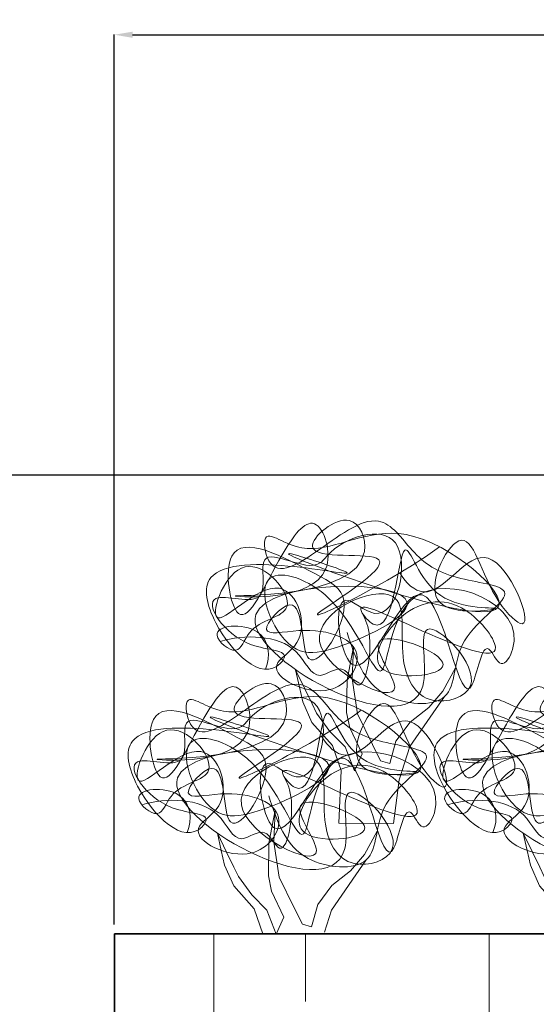
# Model space of a CAD drawing. Units: millimetres. Extents: x -692 to 9639, y -141 to 10345.
# Tile 15 of 19: x 3088 to 3652, y 9272 to 10345. Entities that reach past the tile are written whole.
import ezdxf

# ---------------------------------------------------------------- set-up
doc = ezdxf.new("R2010")
doc.units = ezdxf.units.MM
doc.header["$MEASUREMENT"] = 0
for name, color, linetype, lineweight in [('A-ANNO-DIMS', 2, 'Continuous', 18), ('A-ELEV', 7, 'Continuous', 35), ('A-ELEV-PATT', 8, 'Continuous', 13), ('L-PLNT', 3, 'Continuous', 18)]:
    doc.layers.add(name, color=color, linetype=linetype, lineweight=lineweight)
doc.styles.get("Standard").update_dxf_attribs({"font": 'arial.ttf'})
doc.dimstyles.get("Standard").update_dxf_attribs({"dimtxt": 25, "dimasz": 20, "dimexe": 0.18, "dimexo": 10, "dimgap": 10, "dimtad": 0, "dimtih": 1, "dimtoh": 1, "dimdec": 0, "dimzin": 0, "dimdsep": 46, "dimtxsty": 'Standard', "dimcen": 10, "dimadec": 0, "dimazin": 0, "dimtfac": 1, "dimtdec": 0, "dimtofl": 0, "dimtmove": 0, "dimatfit": 3, "dimfxl": 1, "dimtolj": 1, "dimtzin": 0, "dimarcsym": 0})

# ---------------------------------------------------------------- blocks, each defined once
blk = doc.blocks.new('SHRUB-A')
for p, q in [((56.2, 156.7), (63.1, 192.4)), ((63.1, 192.4), (61.6, 157.6)), ((4.3, 148.6), (0, 167.6)), ((0, 167.6), (10, 146.8)), ((160.6, 144.2), (174.3, 169.5)), ((55.6, 120.9), (56.2, 156.7)), ((61.6, 157.6), (67.3, 119.6)), ((7.9, 132.5), (4.3, 148.6)), ((10, 146.8), (18, 130.3)), ((145.1, 126.5), (160.6, 144.2)), ((17.8, 109.9), (7.9, 132.5)), ((18, 130.3), (22.9, 120.3)), ((162.4, 138.4), (124.4, 83.7)), ((22.9, 120.3), (37.4, 100.1)), ((59.1, 104.1), (55.6, 120.9)), ((67.3, 119.6), (83.9, 86)), ((124.8, 110.5), (145.1, 126.5)), ((40.2, 84.8), (17.8, 109.9)), ((109.4, 89.7), (124.8, 110.5)), ((37.4, 100.1), (54, 83.6)), ((72.4, 75.8), (59.1, 104.1)), ((83.9, 86), (92.7, 68.2)), ((102.6, 65.4), (109.4, 89.7)), ((49.7, 57.7), (40.2, 84.8)), ((54, 83.6), (64.1, 57.4)), ((64.1, 57.4), (72.4, 75.8)), ((124.4, 83.7), (113, 47.4)), ((92.7, 68.2), (102.6, 65.4)), ((47, 0.4), (49.7, 57.7)), ((113, 47.4), (106.7, 0)), ((106.7, 0), (47, 0.4))]:
    blk.add_line(p, q)
blk = doc.blocks.new('SHRUB-B')
for p, q in [((56.2, 99.2), (63.1, 135)), ((63.1, 135), (61.6, 100.2)), ((4.3, 91.2), (0, 110.2)), ((0, 110.2), (10, 89.4)), ((160.6, 86.8), (174.3, 112.1)), ((55.6, 63.5), (56.2, 99.2)), ((61.6, 100.2), (67.3, 62.2)), ((7.9, 75.1), (4.3, 91.2)), ((10, 89.4), (18, 72.9)), ((145.1, 69.1), (160.6, 86.8)), ((17.8, 52.5), (7.9, 75.1)), ((18, 72.9), (22.9, 62.9)), ((124.8, 53.1), (145.1, 69.1)), ((22.9, 62.9), (37.4, 42.7)), ((59.1, 46.7), (55.6, 63.5)), ((67.3, 62.2), (83.9, 28.6)), ((40.2, 27.4), (17.8, 52.5)), ((72.4, 18.4), (59.1, 46.7)), ((109.4, 32.3), (124.8, 53.1)), ((37.4, 42.7), (54, 26.2)), ((102.6, 8), (109.4, 32.3)), ((49.7, 0.3), (40.2, 27.4)), ((54, 26.2), (64.1, 0)), ((83.9, 28.6), (92.7, 10.8)), ((64.1, 0), (72.4, 18.4)), ((92.7, 10.8), (102.6, 8))]:
    blk.add_line(p, q)
blk = doc.blocks.new('*D7')
at = {"layer": 'A-ANNO-DIMS', "color": 0, "lineweight": -2, "transparency": 16777216}
for p, q in [((8481.5, 9848.8), (-649.1, 9848.8)), ((-648.9, 9828.8), (-648.9, 5124.9)), ((-648.9, 375.6), (-648.9, 5079.4)), ((2463.7, 355.6), (-649.1, 355.6))]:
    blk.add_line(p, q, dxfattribs=at)
at = {"layer": 'A-ANNO-DIMS', "color": 0, "lineweight": -3, "transparency": 16777216}
for points in [[(-652.2, 9828.8), (-645.6, 9828.8), (-648.9, 9848.8)], [(-652.2, 375.6), (-645.6, 375.6), (-648.9, 355.6)]]:
    blk.add_solid(points, dxfattribs=at)
at = {"layer": 'Defpoints', "color": 0, "lineweight": -3, "transparency": 16777216}
for p in [(-648.9, 9848.8), (8491.5, 9848.8), (2473.7, 355.6)]:
    blk.add_point(p, dxfattribs=at)
at = {"layer": 'A-ANNO-DIMS', "color": 0, "transparency": 16777216, "insert": (-648.9, 5102.2), "char_height": 25, "attachment_point": 5}
blk.add_mtext('\\A1;9493', dxfattribs=at)
blk = doc.blocks.new('*D14')
at = {"layer": 'A-ANNO-DIMS', "color": 0, "lineweight": -2, "transparency": 16777216}
for p, q in [((3191.5, 9358.8), (3191.5, 10329)), ((3211.5, 10328.8), (4144, 10328.8)), ((5171.5, 10328.8), (4239, 10328.8)), ((5191.5, 9358.8), (5191.5, 10329))]:
    blk.add_line(p, q, dxfattribs=at)
at = {"layer": 'A-ANNO-DIMS', "color": 0, "lineweight": -3, "transparency": 16777216}
for points in [[(3211.5, 10332.1), (3211.5, 10325.4), (3191.5, 10328.8)], [(5171.5, 10332.1), (5171.5, 10325.4), (5191.5, 10328.8)]]:
    blk.add_solid(points, dxfattribs=at)
at = {"layer": 'Defpoints', "color": 0, "lineweight": -3, "transparency": 16777216}
for p in [(5191.5, 10328.8), (3191.5, 9348.8), (5191.5, 9348.8)]:
    blk.add_point(p, dxfattribs=at)
at = {"layer": 'A-ANNO-DIMS', "color": 0, "transparency": 16777216, "insert": (4191.5, 10328.8), "char_height": 25, "attachment_point": 5}
blk.add_mtext('\\A1;2000', dxfattribs=at)

msp = doc.modelspace()

# ---------------------------------------------------------------- hatches: boundary and pattern name
at = {"layer": 'A-ELEV-PATT'}
h = msp.add_hatch(dxfattribs=at)
h.set_pattern_fill('GOST_WOOD', color=256, scale=50)
h.set_pattern_definition([(90, (0, 0), (300, -2e-14), [500, -100]), (90, (100, -100), (300, -2e-14), [300, -75, 150, -75]), (90, (200, -250), (300, -2e-14), [500, -100])])
edge = h.paths.add_edge_path()
edge.add_line((5191.547, 8748.772), (3791.547, 8748.772))
edge.add_line((3791.547, 8748.772), (3791.547, 8848.772))
edge.add_line((3791.547, 8848.772), (5191.547, 8848.772))
edge.add_line((5191.547, 8848.772), (5191.547, 9348.772))
edge.add_line((5191.547, 9348.772), (4755.992, 9348.772))
edge.add_line((4755.992, 9348.772), (4755.854, 9348.465))
edge.add_line((4755.854, 9348.465), (4755.734, 9348.772))
edge.add_line((4755.734, 9348.772), (4053.129, 9348.772))
edge.add_line((4053.129, 9348.772), (4052.99, 9348.465))
edge.add_line((4052.99, 9348.465), (4052.871, 9348.772))
edge.add_line((4052.871, 9348.772), (3701.731, 9348.772))
edge.add_line((3701.731, 9348.772), (3701.593, 9348.465))
edge.add_line((3701.593, 9348.465), (3701.474, 9348.772))
edge.add_line((3701.474, 9348.772), (3368.199, 9348.772))
edge.add_line((3368.199, 9348.772), (3368.061, 9348.465))
edge.add_line((3368.061, 9348.465), (3367.942, 9348.772))
edge.add_line((3367.942, 9348.772), (3191.547, 9348.772))
edge.add_line((3191.547, 9348.772), (3191.547, 3210.058))
edge.add_spline(control_points=[(3191.547, 3210.058), (3198.467, 3207.5), (3283.859, 3166.656), (3324.053, 2995.08), (3234.02, 2920.058), (3220.783, 2911.684)], knot_values=[13649.89756952, 13649.89756952, 13649.89756952, 13649.89756952, 13672.14990348, 13935.42377748, 13974.4426778, 13974.4426778, 13974.4426778, 13974.4426778], degree=3, periodic=0)
edge.add_spline(control_points=[(3220.783, 2911.684), (3225.148, 2890.107), (3226.864, 2868.931), (3226.144, 2848.27)], knot_values=[8828.69997321, 8828.69997321, 8828.69997321, 8828.69997321, 8890.6429847, 8890.6429847, 8890.6429847, 8890.6429847], degree=3, periodic=0)
edge.add_line((3226.144, 2848.27), (5191.547, 2848.27))
edge.add_line((5191.547, 2848.27), (5191.547, 3048.27))
edge.add_line((5191.547, 3048.27), (5041.547, 3048.27))
edge.add_line((5041.547, 3048.27), (5041.547, 3148.27))
edge.add_line((5041.547, 3148.27), (5091.547, 3148.27))
edge.add_line((5091.547, 3148.27), (5091.547, 3598.27))
edge.add_line((5091.547, 3598.27), (5191.547, 3598.27))
edge.add_line((5191.547, 3598.27), (5191.547, 4848.772))
edge.add_line((5191.547, 4848.772), (3791.547, 4848.772))
edge.add_line((3791.547, 4848.772), (3791.547, 6848.772))
edge.add_line((3791.547, 6848.772), (5091.547, 6848.772))
edge.add_line((5091.547, 6848.772), (5091.547, 7298.772))
edge.add_line((5091.547, 7298.772), (5191.547, 7298.772))
edge.add_line((5191.547, 7298.772), (5191.547, 8748.772))
h.paths.add_polyline_path([(5016.547, 8198.772), (5016.547, 7123.772), (3941.547, 7123.772), (3941.547, 8198.772)], flags=16)
h.paths.add_polyline_path([(4941.547, 8123.772), (4941.547, 7198.772), (4016.547, 7198.772), (4016.547, 8123.772)], flags=0)
h.paths.add_polyline_path([(4616.547, 8073.772), (4616.547, 7248.772), (4341.547, 7248.772), (4341.547, 8073.772)], flags=0)
h.paths.add_polyline_path([(4641.547, 8073.772), (4891.547, 8073.772), (4891.547, 7248.772), (4641.547, 7248.772)], flags=0)
h.paths.add_polyline_path([(4666.547, 8048.772), (4866.547, 8048.772), (4866.547, 7273.772), (4666.547, 7273.772)], flags=0)
h.paths.add_polyline_path([(4316.547, 8073.772), (4316.547, 7248.772), (4066.547, 7248.772), (4066.547, 8073.772)], flags=0)
h.paths.add_polyline_path([(4291.547, 8048.772), (4291.547, 7273.772), (4091.547, 7273.772), (4091.547, 8048.772)], flags=0)
h.paths.add_polyline_path([(5016.547, 4497.772), (5016.547, 3422.772), (3941.547, 3422.772), (3941.547, 4497.772)], flags=16)
h.paths.add_polyline_path([(4941.547, 4422.772), (4941.547, 3497.772), (4016.547, 3497.772), (4016.547, 4422.772)], flags=0)
h.paths.add_polyline_path([(4616.547, 4372.772), (4616.547, 3547.772), (4341.547, 3547.772), (4341.547, 4372.772)], flags=0)
h.paths.add_polyline_path([(4641.547, 4372.772), (4891.547, 4372.772), (4891.547, 3547.772), (4641.547, 3547.772)], flags=0)
h.paths.add_polyline_path([(4316.547, 4372.772), (4316.547, 3547.772), (4066.547, 3547.772), (4066.547, 4372.772)], flags=0)
h.paths.add_polyline_path([(4666.547, 4347.772), (4866.547, 4347.772), (4866.547, 3572.772), (4666.547, 3572.772)], flags=0)
h.paths.add_polyline_path([(4291.547, 4347.772), (4291.547, 3572.772), (4091.547, 3572.772), (4091.547, 4347.772)], flags=0)

# ---------------------------------------------------------------- linework, layer by layer
at = {"layer": 'A-ELEV'}
for p, q in [((3191.547, 2848.27), (3191.547, 9348.772)), ((3191.547, 9348.772), (5191.547, 9348.772))]:
    msp.add_line(p, q, dxfattribs=at)
at = {"layer": 'L-PLNT'}
for p, q in [((3466.365, 9429.44), (3428.3, 9374.709)), ((3428.3, 9374.709), (3420.723, 9350.541))]:
    msp.add_line(p, q, dxfattribs=at)
for points, knots in [([(3502.938, 9742.239), (3509.443, 9730.903), (3542.679, 9700.951), (3599.109, 9812.559), (3658.29, 9660.867), (3593.653, 9722.363), (3577.928, 9821.568), (3510.969, 9687.955), (3648.435, 9708.276), (3531.59, 9697.909), (3502.254, 9822.951), (3496.652, 9656.273), (3444.15, 9718.176), (3537.831, 9672.588), (3634.897, 9634.5), (3565.736, 9723.816), (3499.582, 9704.087), (3457.371, 9620.458), (3608.259, 9634.855), (3442.65, 9696.668), (3539.024, 9576.858), (3345.182, 9670.533), (3519.878, 9749.582), (3497.67, 9651.408), (3526.407, 9592.145), (3612.659, 9617.027), (3510.825, 9721.539), (3566.031, 9522.359), (3180.437, 9733.486), (3595.531, 9736.751), (3445.548, 9659.817), (3374.696, 9649.423), (3331.884, 9757.262), (3446.665, 9723.536), (3488.753, 9579.097), (3493.738, 9768.661), (3655.432, 9702.629), (3612.705, 9633.263), (3594.668, 9680.84), (3573.873, 9544.945), (3537.119, 9826.86), (3449.988, 9563.572), (3424.986, 9739.876), (3494.755, 9668.929), (3526.422, 9809.339), (3435.881, 9778.979), (3406.756, 9737.949), (3339.813, 9784.348), (3366.004, 9697.774), (3273.562, 9733.91), (3323.379, 9654.8), (3384.898, 9658.957), (3354.732, 9620.328), (3299.428, 9675.174), (3275.146, 9782.065), (3519.521, 9719.852), (3271.229, 9801.027), (3731.978, 9622.054), (3506.313, 9821.297), (3426.47, 9760.575), (3380.167, 9773.261), (3352.083, 9789.116), (3364.445, 9699.252), (3465.774, 9839.527), (3517.913, 9759.776), (3556.728, 9734.293), (3648.404, 9726.404), (3555.387, 9674.075), (3569.548, 9593.308), (3469.73, 9601.408), (3454.103, 9650.09), (3445.36, 9677.329)], [2413.81083439, 2413.81083439, 2413.81083439, 2413.81083439, 2446.13175162, 2525.76080664, 2606.35842411, 2641.00152553, 2720.74212251, 2790.99014926, 2851.81652626, 2913.32865241, 2976.26621652, 3063.90114016, 3082.75198237, 3142.42040078, 3234.21047015, 3290.89514405, 3366.44484787, 3415.98940505, 3483.69911772, 3557.93307926, 3609.73318023, 3705.73947781, 3799.4035149, 3865.9559372, 3923.0506034, 3967.47996902, 4044.49288828, 4106.44083814, 4304.51898163, 4470.20683119, 4567.66187689, 4605.3795614, 4686.71522755, 4750.59418277, 4853.67923318, 4940.38216709, 5061.92671957, 5081.75583403, 5102.38342504, 5145.20608443, 5257.20859169, 5364.77120979, 5434.601162, 5468.93345211, 5548.91442162, 5624.29444335, 5636.24531967, 5696.20028889, 5735.53268567, 5783.76480276, 5846.42206129, 5886.03768999, 5892.5373904, 5975.51315878, 6025.10951571, 6171.93373357, 6229.50952465, 6457.88730992, 6585.61219414, 6694.59236697, 6720.94216912, 6740.48817363, 6762.80712224, 6890.45590486, 6938.76737224, 6996.52597549, 7050.2147859, 7119.04318667, 7183.57042671, 7247.02609863, 7327.63038966, 7327.63038966, 7327.63038966, 7327.63038966]), ([(3356.247, 9637.137), (3362.31, 9651.341), (3358.815, 9689.445), (3284.244, 9684.583), (3327.692, 9647.305), (3338.373, 9691.38), (3407.434, 9694.456), (3327.482, 9786.768), (3278.987, 9649.897), (3377.462, 9765.156), (3409.237, 9667.558), (3345.184, 9636.75), (3427.987, 9595.485), (3475.333, 9663.04), (3410.887, 9686.864), (3340.346, 9669.411), (3401.85, 9738.522), (3388.906, 9597.689), (3463.217, 9714.368), (3397.453, 9747.322), (3301.678, 9801.44), (3325.843, 9656.882), (3365.416, 9753.527), (3412.553, 9818.105), (3446.144, 9708.231), (3217.396, 9723.215), (3491.544, 9710.208), (3451.543, 9819.441), (3368.144, 9748.74), (3543.178, 9777.439), (3331.654, 9652.419), (3495.907, 9733.103), (3546.039, 9770.678)], [369.05069933, 369.05069933, 369.05069933, 369.05069933, 408.0755152, 451.81999766, 477.70991819, 501.76804774, 551.72688153, 614.71506468, 677.59190345, 752.65992621, 814.92518896, 848.06947292, 911.78367098, 957.89252981, 1028.01014559, 1063.15062915, 1099.93333455, 1162.00574744, 1235.23981988, 1278.45742209, 1371.86548038, 1434.47491944, 1513.90135623, 1562.79289697, 1613.81915843, 1716.27616866, 1864.9556669, 1902.31221643, 1951.61463942, 2025.20033993, 2111.30740148, 2244.75178922, 2244.75178922, 2244.75178922, 2244.75178922]), ([(3460.967, 9700.071), (3464.458, 9693.404), (3475.954, 9671.444), (3462.883, 9597.516), (3441.702, 9646.949), (3408.892, 9618.501), (3391.305, 9674.749), (3333.552, 9675.405), (3306.841, 9667.541)], [0, 0, 0, 0, 24.87287104, 81.92705424, 103.09014331, 128.64171207, 165.87657864, 231.33124244, 231.33124244, 231.33124244, 231.33124244]), ([(3417.588, 9564.196), (3424.093, 9552.861), (3457.329, 9522.909), (3513.759, 9634.516), (3572.939, 9482.824), (3508.303, 9544.32), (3492.577, 9643.525), (3425.618, 9509.913), (3563.084, 9530.233), (3446.24, 9519.866), (3416.904, 9644.908), (3411.302, 9478.231), (3358.8, 9540.133), (3452.481, 9494.545), (3549.546, 9456.457), (3480.385, 9545.773), (3414.232, 9526.044), (3372.021, 9442.416), (3522.909, 9456.812), (3357.3, 9518.625), (3453.674, 9398.815), (3259.832, 9492.49), (3434.528, 9571.539), (3412.319, 9473.365), (3441.057, 9414.102), (3527.309, 9438.984), (3425.475, 9543.496), (3480.681, 9344.316), (3095.087, 9555.443), (3510.181, 9558.708), (3360.198, 9481.774), (3289.346, 9471.381), (3246.534, 9579.22), (3361.315, 9545.493), (3403.403, 9401.054), (3408.388, 9590.618), (3570.081, 9524.586), (3527.354, 9455.22), (3509.317, 9502.798), (3488.522, 9366.902), (3451.769, 9648.817), (3364.638, 9385.529), (3339.636, 9561.834), (3409.405, 9490.886), (3441.071, 9631.296), (3350.531, 9600.937), (3321.405, 9559.906), (3254.463, 9606.306), (3280.654, 9519.731), (3188.212, 9555.867), (3238.029, 9476.758), (3299.548, 9480.914), (3269.382, 9442.286), (3214.078, 9497.131), (3189.796, 9604.022), (3434.17, 9541.809), (3185.879, 9622.984), (3646.628, 9444.011), (3420.963, 9643.254), (3341.119, 9582.532), (3294.817, 9595.218), (3266.733, 9611.073), (3279.095, 9521.209), (3380.423, 9661.484), (3432.563, 9581.734), (3471.377, 9556.25), (3563.053, 9548.361), (3470.036, 9496.032), (3484.197, 9415.265), (3384.38, 9423.365), (3368.753, 9472.047), (3360.01, 9499.286)], [2413.81083439, 2413.81083439, 2413.81083439, 2413.81083439, 2446.13175162, 2525.76080664, 2606.35842411, 2641.00152553, 2720.74212251, 2790.99014926, 2851.81652626, 2913.32865241, 2976.26621652, 3063.90114016, 3082.75198237, 3142.42040078, 3234.21047015, 3290.89514405, 3366.44484787, 3415.98940505, 3483.69911772, 3557.93307926, 3609.73318023, 3705.73947781, 3799.4035149, 3865.9559372, 3923.0506034, 3967.47996902, 4044.49288828, 4106.44083814, 4304.51898163, 4470.20683119, 4567.66187689, 4605.3795614, 4686.71522755, 4750.59418277, 4853.67923318, 4940.38216709, 5061.92671957, 5081.75583403, 5102.38342504, 5145.20608443, 5257.20859169, 5364.77120979, 5434.601162, 5468.93345211, 5548.91442162, 5624.29444335, 5636.24531967, 5696.20028889, 5735.53268567, 5783.76480276, 5846.42206129, 5886.03768999, 5892.5373904, 5975.51315878, 6025.10951571, 6171.93373357, 6229.50952465, 6457.88730992, 6585.61219414, 6694.59236697, 6720.94216912, 6740.48817363, 6762.80712224, 6890.45590486, 6938.76737224, 6996.52597549, 7050.2147859, 7119.04318667, 7183.57042671, 7247.02609863, 7327.63038966, 7327.63038966, 7327.63038966, 7327.63038966]), ([(3751.119, 9564.196), (3757.625, 9552.861), (3790.861, 9522.909), (3847.291, 9634.516), (3906.471, 9482.824), (3841.835, 9544.32), (3826.109, 9643.525), (3759.15, 9509.913), (3896.616, 9530.233), (3779.772, 9519.866), (3750.436, 9644.908), (3744.834, 9478.231), (3692.332, 9540.133), (3786.013, 9494.545), (3883.078, 9456.457), (3813.917, 9545.773), (3747.764, 9526.044), (3705.553, 9442.416), (3856.44, 9456.812), (3690.831, 9518.625), (3787.206, 9398.815), (3593.364, 9492.49), (3768.06, 9571.539), (3745.851, 9473.365), (3774.589, 9414.102), (3860.841, 9438.984), (3759.007, 9543.496), (3814.213, 9344.316), (3428.619, 9555.443), (3843.713, 9558.708), (3693.73, 9481.774), (3622.878, 9471.381), (3580.065, 9579.22), (3694.847, 9545.493), (3736.934, 9401.054), (3741.92, 9590.618), (3903.613, 9524.586), (3860.886, 9455.22), (3842.849, 9502.798), (3822.054, 9366.902), (3785.301, 9648.817), (3698.169, 9385.529), (3673.168, 9561.834), (3742.936, 9490.886), (3774.603, 9631.296), (3684.063, 9600.937), (3654.937, 9559.906), (3587.995, 9606.306), (3614.186, 9519.731), (3521.744, 9555.867), (3571.56, 9476.758), (3633.08, 9480.914), (3602.913, 9442.286), (3547.609, 9497.131), (3523.328, 9604.022), (3767.702, 9541.809), (3519.41, 9622.984), (3980.16, 9444.011), (3754.495, 9643.254), (3674.651, 9582.532), (3628.349, 9595.218), (3600.265, 9611.073), (3612.627, 9521.209), (3713.955, 9661.484), (3766.095, 9581.734), (3804.909, 9556.25), (3896.585, 9548.361), (3803.568, 9496.032), (3817.729, 9415.265), (3717.911, 9423.365), (3702.285, 9472.047), (3693.541, 9499.286)], [2413.81083439, 2413.81083439, 2413.81083439, 2413.81083439, 2446.13175162, 2525.76080664, 2606.35842411, 2641.00152553, 2720.74212251, 2790.99014926, 2851.81652626, 2913.32865241, 2976.26621652, 3063.90114016, 3082.75198237, 3142.42040078, 3234.21047015, 3290.89514405, 3366.44484787, 3415.98940505, 3483.69911772, 3557.93307926, 3609.73318023, 3705.73947781, 3799.4035149, 3865.9559372, 3923.0506034, 3967.47996902, 4044.49288828, 4106.44083814, 4304.51898163, 4470.20683119, 4567.66187689, 4605.3795614, 4686.71522755, 4750.59418277, 4853.67923318, 4940.38216709, 5061.92671957, 5081.75583403, 5102.38342504, 5145.20608443, 5257.20859169, 5364.77120979, 5434.601162, 5468.93345211, 5548.91442162, 5624.29444335, 5636.24531967, 5696.20028889, 5735.53268567, 5783.76480276, 5846.42206129, 5886.03768999, 5892.5373904, 5975.51315878, 6025.10951571, 6171.93373357, 6229.50952465, 6457.88730992, 6585.61219414, 6694.59236697, 6720.94216912, 6740.48817363, 6762.80712224, 6890.45590486, 6938.76737224, 6996.52597549, 7050.2147859, 7119.04318667, 7183.57042671, 7247.02609863, 7327.63038966, 7327.63038966, 7327.63038966, 7327.63038966]), ([(3270.897, 9459.094), (3276.96, 9473.298), (3273.465, 9511.403), (3198.894, 9506.54), (3242.341, 9469.262), (3253.023, 9513.337), (3322.084, 9516.414), (3242.132, 9608.725), (3193.637, 9471.854), (3292.112, 9587.113), (3323.887, 9489.516), (3259.834, 9458.707), (3342.637, 9417.442), (3389.983, 9484.997), (3325.537, 9508.821), (3254.996, 9491.368), (3316.5, 9560.479), (3303.555, 9419.646), (3377.867, 9536.325), (3312.103, 9569.279), (3216.327, 9623.397), (3240.492, 9478.839), (3280.066, 9575.484), (3327.202, 9640.062), (3360.793, 9530.189), (3132.045, 9545.172), (3406.194, 9532.166), (3366.192, 9641.398), (3282.793, 9570.697), (3457.828, 9599.396), (3246.304, 9474.376), (3410.557, 9555.06), (3460.689, 9592.636)], [369.05069933, 369.05069933, 369.05069933, 369.05069933, 408.0755152, 451.81999766, 477.70991819, 501.76804774, 551.72688153, 614.71506468, 677.59190345, 752.65992621, 814.92518896, 848.06947292, 911.78367098, 957.89252981, 1028.01014559, 1063.15062915, 1099.93333455, 1162.00574744, 1235.23981988, 1278.45742209, 1371.86548038, 1434.47491944, 1513.90135623, 1562.79289697, 1613.81915843, 1716.27616866, 1864.9556669, 1902.31221643, 1951.61463942, 2025.20033993, 2111.30740148, 2244.75178922, 2244.75178922, 2244.75178922, 2244.75178922]), ([(3604.428, 9459.094), (3610.491, 9473.298), (3606.997, 9511.403), (3532.426, 9506.54), (3575.873, 9469.262), (3586.555, 9513.337), (3655.616, 9516.414), (3575.664, 9608.725), (3527.168, 9471.854), (3625.644, 9587.113), (3657.419, 9489.516), (3593.366, 9458.707), (3676.168, 9417.442), (3723.515, 9484.997), (3659.069, 9508.821), (3588.527, 9491.368), (3650.032, 9560.479), (3637.087, 9419.646), (3711.399, 9536.325), (3645.635, 9569.279), (3549.859, 9623.397), (3574.024, 9478.839), (3613.598, 9575.484), (3660.734, 9640.062), (3694.325, 9530.189), (3465.577, 9545.172), (3739.726, 9532.166), (3699.724, 9641.398), (3616.325, 9570.697), (3791.36, 9599.396), (3579.836, 9474.376), (3744.089, 9555.06), (3794.22, 9592.636)], [369.05069933, 369.05069933, 369.05069933, 369.05069933, 408.0755152, 451.81999766, 477.70991819, 501.76804774, 551.72688153, 614.71506468, 677.59190345, 752.65992621, 814.92518896, 848.06947292, 911.78367098, 957.89252981, 1028.01014559, 1063.15062915, 1099.93333455, 1162.00574744, 1235.23981988, 1278.45742209, 1371.86548038, 1434.47491944, 1513.90135623, 1562.79289697, 1613.81915843, 1716.27616866, 1864.9556669, 1902.31221643, 1951.61463942, 2025.20033993, 2111.30740148, 2244.75178922, 2244.75178922, 2244.75178922, 2244.75178922]), ([(3375.617, 9522.028), (3379.107, 9515.361), (3390.604, 9493.402), (3377.533, 9419.473), (3356.352, 9468.907), (3323.542, 9440.458), (3305.955, 9496.706), (3248.202, 9497.363), (3221.49, 9489.498)], [0, 0, 0, 0, 24.87287104, 81.92705424, 103.09014331, 128.64171207, 165.87657864, 231.33124244, 231.33124244, 231.33124244, 231.33124244]), ([(3709.149, 9522.028), (3712.639, 9515.361), (3724.136, 9493.402), (3711.065, 9419.473), (3689.884, 9468.907), (3657.074, 9440.458), (3639.487, 9496.706), (3581.734, 9497.363), (3555.022, 9489.498)], [0, 0, 0, 0, 24.87287104, 81.92705424, 103.09014331, 128.64171207, 165.87657864, 231.33124244, 231.33124244, 231.33124244, 231.33124244])]:
    msp.add_open_spline(points, degree=3, knots=knots, dxfattribs=at)

# ---------------------------------------------------------------- block references
for name, p in [('SHRUB-A', (3389.269, 9469.1)), ('SHRUB-B', (3303.919, 9348.465)), ('SHRUB-B', (3637.451, 9348.465))]:
    msp.add_blockref(name, p, dxfattribs=at)

# ---------------------------------------------------------------- dimensions: what is measured, and where the dimension line sits
at = {"layer": 'A-ANNO-DIMS'}
dim = msp.add_linear_dim(base=(5191.547, 10328.772), p1=(3191.547, 9348.772), p2=(5191.547, 9348.772), dimstyle='Standard', override={"dimdec": 0, "dimlfac": 1, "dimrnd": 0, "dimzin": 0, "dimdsep": 46, "dimlunit": 2}, dxfattribs=at)
dim.commit()
dim.dimension.update_dxf_attribs({"geometry": '*D14', "text_midpoint": (4191.547, 10328.772)})
dim = msp.add_linear_dim(base=(-648.912, 9848.772), p1=(2473.746, 355.575), p2=(8491.547, 9848.772), angle=90, dimstyle='Standard', override={"dimdec": 0, "dimlfac": 1, "dimrnd": 0, "dimzin": 0, "dimdsep": 46, "dimlunit": 2}, dxfattribs=at)
dim.commit()
dim.dimension.update_dxf_attribs({"geometry": '*D7', "text_midpoint": (-648.912, 5102.173)})

doc.saveas('drawing.dxf')
